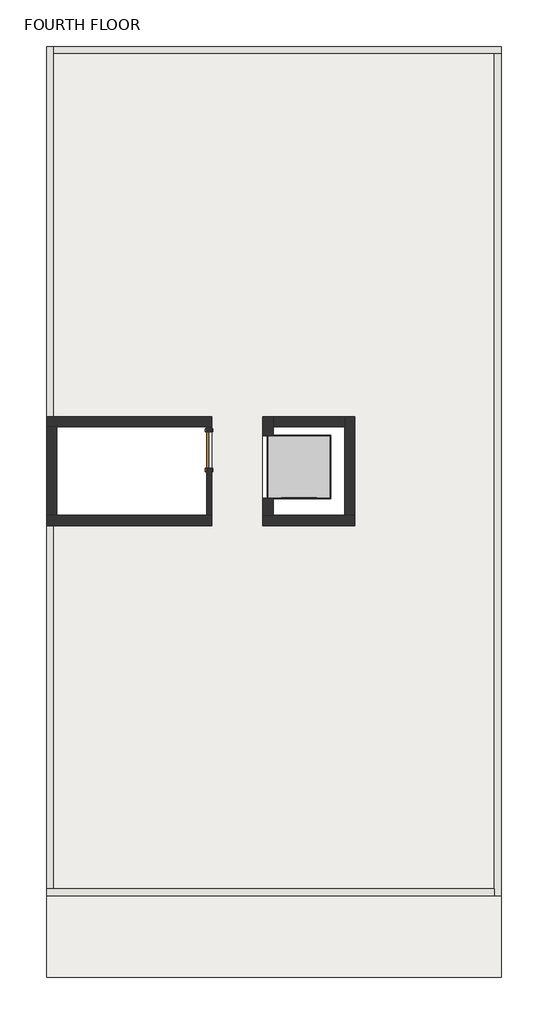
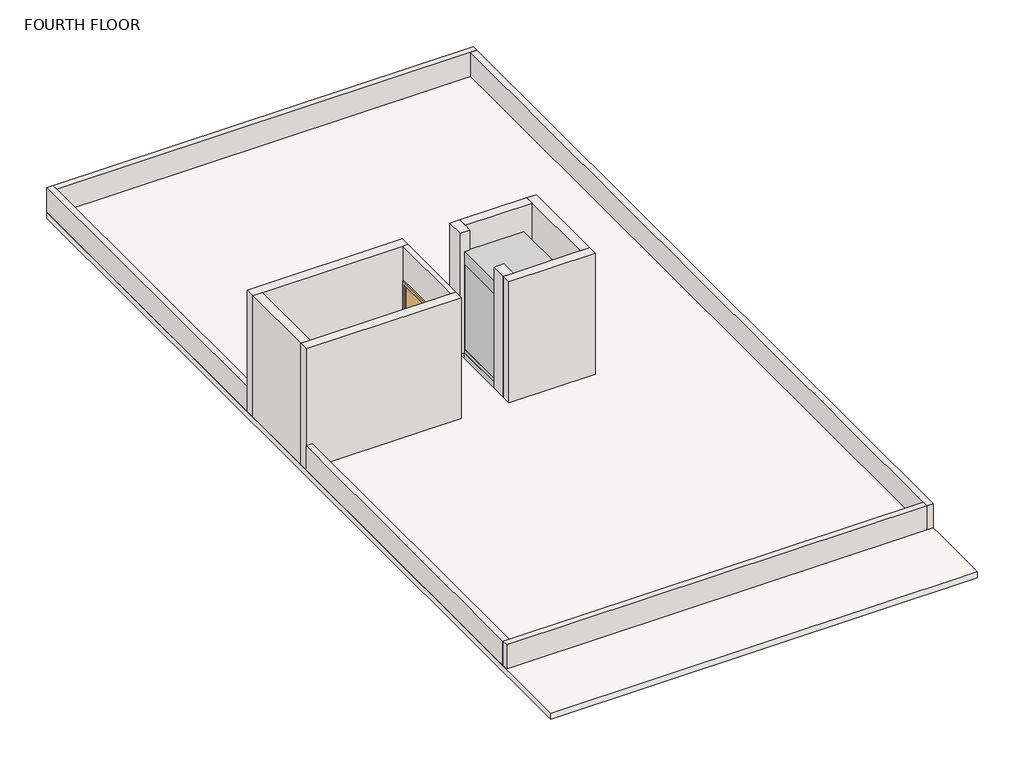
# One storey, incomplete: 14 walls, 1 door, 1 proxy, 1 slab.
"""IFC4 building model written with IfcOpenShell, lengths in millimetres."""

from ifc_helpers import new_model, si_unit, frame, origin, place, context, project, spatial, polyline, outline, extrude, faceted_brep, transform, mapped, element, save
from components import lift_glass_2_lift_with_hydraulic_ram_a28bd677, door_d141acb4

model = new_model("IFC4")

# Units and contexts
model_context = context("Model", 3, world=origin())
ifc_project = project(units=[si_unit("LENGTHUNIT", "METRE", prefix="MILLI")], contexts=[model_context])

# Site, building, storey
site = spatial("IfcSite", under=ifc_project)
building = spatial("IfcBuilding", under=site)
storey = spatial("IfcBuildingStorey", under=building, Name="FOURTH FLOOR", Elevation=12801.6)

# Proxy
placement = place(None, origin())
lift_glass_2_lift_with_hydraulic_ram_shape = lift_glass_2_lift_with_hydraulic_ram_a28bd677(model_context)
element("IfcBuildingElementProxy", 1, Name="Lift Glass (2) : Lift with Hydraulic Ram", ObjectType="Lift Glass (2) : Lift with Hydraulic Ram", at=placement, inside=storey, context=model_context, shape_type="MappedRepresentation", body=[
    mapped(lift_glass_2_lift_with_hydraulic_ram_shape, transform((-743.7147577, 597.8900134, 12801.6), x_axis=(1.0, 0.0, 0.0), y_axis=(0.0, 1.0, 0.0), z_axis=(0.0, 0.0, 1.0))),
])

# Door
door_shape = door_d141acb4(model_context)
element("IfcDoor", 2, ObjectType="Single-Flush : 2'8\"X7'", at=placement, inside=storey, context=model_context, shape_type="MappedRepresentation", body=[
    mapped(door_shape, transform((-2719.6789041, 1029.1153263, 12801.6), x_axis=(0.0, 1.0, 0.0), y_axis=(-1.0, 0.0, 0.0), z_axis=(0.0, 0.0, 1.0))),
])

# Slab
element("IfcSlab", 3, ObjectType="6\"", at=placement, inside=storey, context=model_context, shape_type="SweptSolid", body=[
    extrude(outline(polyline([(3814.4710959, 10058.8153263), (3814.4710959, -10769.1846737), (-6358.2289041, -10769.1846737), (-6358.2289041, 10058.8153263), (3814.4710959, 10058.8153263)]), holes=[polyline([(-2662.5289041, 1549.8153263), (-6129.6289041, 1549.8153263), (-6129.6289041, -431.3846737), (-2662.5289041, -431.3846737), (-2662.5289041, 1549.8153263)]), polyline([(537.8710959, 1778.4153263), (-1519.5289041, 1778.4153263), (-1519.5289041, -659.9846737), (537.8710959, -659.9846737), (537.8710959, 1778.4153263)])]), frame((0.0, 0.0, 12649.2), z_axis=(0.0, 0.0, 1.0), x_axis=(1.0, 0.0, 0.0)), (0.0, 0.0, 1.0), 152.4),
])

# Walls
element("IfcWall", 4, ObjectType="4.5\"", at=placement, inside=storey, context=model_context, shape_type="SweptSolid", body=[
    extrude(outline(polyline([(1549.8153263, 12801.6), (1435.5153263, 12801.6), (1435.5153263, 14935.2), (622.7153263, 14935.2), (622.7153263, 12801.6), (-431.3846737, 12801.6), (-431.3846737, 15849.6), (1549.8153263, 15849.6), (1549.8153263, 12801.6)])), frame((-2776.8289041, 0.0, 0.0), z_axis=(1.0, 0.0, 0.0), x_axis=(0.0, 1.0, 0.0)), (0.0, 0.0, 1.0), 114.3),
])
element("IfcWall", 5, ObjectType="6\"", at=placement, inside=storey, context=model_context, shape_type="Brep", body=[
    faceted_brep([(-6205.8289041, 1778.4153263, 12801.6), (-6205.8289041, 9906.4153263, 12801.6), (-6205.8289041, 10058.8153263, 12801.6), (-6205.8289041, 10058.8153263, 13411.2), (-6205.8289041, 9906.4153263, 13411.2), (-6205.8289041, 1778.4153263, 13411.2), (-6358.2289041, 1778.4153263, 12801.6), (-6358.2289041, 1778.4153263, 13411.2), (-6358.2289041, 10058.8153263, 13411.2), (-6358.2289041, 10058.8153263, 12801.6)], [[[0, 1, 2, 3, 4, 5]], [[6, 7, 8, 9]], [[2, 1, 0, 6, 9]], [[5, 4, 3, 8, 7]], [[0, 5, 7, 6]], [[3, 2, 9, 8]]]),
])
element("IfcWall", 6, ObjectType="6\"", at=placement, inside=storey, context=model_context, shape_type="Brep", body=[
    faceted_brep([(-6205.8289041, 9906.4153263, 12801.6), (3662.0710959, 9906.4153263, 12801.6), (3814.4710959, 9906.4153263, 12801.6), (3814.4710959, 9906.4153263, 13411.2), (3662.0710959, 9906.4153263, 13411.2), (-6205.8289041, 9906.4153263, 13411.2), (-6205.8289041, 10058.8153263, 12801.6), (-6205.8289041, 10058.8153263, 13411.2), (3814.4710959, 10058.8153263, 13411.2), (3814.4710959, 10058.8153263, 12801.6)], [[[0, 1, 2, 3, 4, 5]], [[6, 7, 8, 9]], [[2, 1, 0, 6, 9]], [[5, 4, 3, 8, 7]], [[0, 5, 7, 6]], [[3, 2, 9, 8]]]),
])
element("IfcWall", 7, ObjectType="6\"", at=placement, inside=storey, context=model_context, shape_type="Brep", body=[
    faceted_brep([(3662.0710959, 9906.4153263, 12801.6), (3662.0710959, -8787.9846737, 12801.6), (3662.0710959, -8940.3846737, 12801.6), (3662.0710959, -8940.3846737, 13411.2), (3662.0710959, -8787.9846737, 13411.2), (3662.0710959, 9906.4153263, 13411.2), (3814.4710959, 9906.4153263, 12801.6), (3814.4710959, 9906.4153263, 13411.2), (3814.4710959, -8940.3846737, 13411.2), (3814.4710959, -8940.3846737, 12801.6)], [[[0, 1, 2, 3, 4, 5]], [[6, 7, 8, 9]], [[2, 1, 0, 6, 9]], [[5, 4, 3, 8, 7]], [[0, 5, 7, 6]], [[3, 2, 9, 8]]]),
])
element("IfcWall", 8, ObjectType="6\"", at=placement, inside=storey, context=model_context, shape_type="Brep", body=[
    faceted_brep([(3662.0710959, -8787.9846737, 12801.6), (-6205.8289041, -8787.9846737, 12801.6), (-6358.2289041, -8787.9846737, 12801.6), (-6358.2289041, -8787.9846737, 13411.2), (-6205.8289041, -8787.9846737, 13411.2), (3662.0710959, -8787.9846737, 13411.2), (3662.0710959, -8940.3846737, 12801.6), (3662.0710959, -8940.3846737, 13411.2), (-6358.2289041, -8940.3846737, 13411.2), (-6358.2289041, -8940.3846737, 12801.6)], [[[0, 1, 2, 3, 4, 5]], [[6, 7, 8, 9]], [[2, 1, 0, 6, 9]], [[5, 4, 3, 8, 7]], [[0, 5, 7, 6]], [[3, 2, 9, 8]]]),
])
element("IfcWall", 9, ObjectType="6\"", at=placement, inside=storey, context=model_context, shape_type="SweptSolid", body=[
    extrude(outline(polyline([(-6205.8289041, -659.9846737), (-6205.8289041, -8787.9846737), (-6358.2289041, -8787.9846737), (-6358.2289041, -659.9846737), (-6205.8289041, -659.9846737)])), frame((0.0, 0.0, 12801.6), z_axis=(0.0, 0.0, 1.0), x_axis=(1.0, 0.0, 0.0)), (0.0, 0.0, 1.0), 609.6),
])
element("IfcWall", 10, ObjectType="9\"", at=placement, inside=storey, context=model_context, shape_type="Brep", body=[
    faceted_brep([(-2662.5289041, 1778.4153263, 12801.6), (-6205.8289041, 1778.4153263, 12801.6), (-6358.2289041, 1778.4153263, 12801.6), (-6358.2289041, 1778.4153263, 13411.2), (-6358.2289041, 1778.4153263, 15849.6), (-2662.5289041, 1778.4153263, 15849.6), (-2662.5289041, 1549.8153263, 12801.6), (-2662.5289041, 1549.8153263, 15849.6), (-2776.8289041, 1549.8153263, 15849.6), (-6129.6289041, 1549.8153263, 15849.6), (-6358.2289041, 1549.8153263, 15849.6), (-6358.2289041, 1549.8153263, 12801.6), (-6129.6289041, 1549.8153263, 12801.6), (-2776.8289041, 1549.8153263, 12801.6)], [[[0, 1, 2, 3, 4, 5]], [[6, 7, 8, 9, 10, 11, 12, 13]], [[2, 1, 0, 6, 13, 12, 11]], [[5, 4, 10, 9, 8, 7]], [[0, 5, 7, 6]], [[2, 11, 10, 4, 3]]]),
])
element("IfcWall", 11, ObjectType="9\"", at=placement, inside=storey, context=model_context, shape_type="Brep", body=[
    faceted_brep([(-2662.5289041, -431.3846737, 12801.6), (-2776.8289041, -431.3846737, 12801.6), (-6129.6289041, -431.3846737, 12801.6), (-6358.2289041, -431.3846737, 12801.6), (-6358.2289041, -431.3846737, 15849.6), (-6129.6289041, -431.3846737, 15849.6), (-2776.8289041, -431.3846737, 15849.6), (-2662.5289041, -431.3846737, 15849.6), (-2662.5289041, -659.9846737, 12801.6), (-2662.5289041, -659.9846737, 15849.6), (-6358.2289041, -659.9846737, 15849.6), (-6358.2289041, -659.9846737, 13411.2), (-6358.2289041, -659.9846737, 12801.6), (-6205.8289041, -659.9846737, 12801.6)], [[[0, 1, 2, 3, 4, 5, 6, 7]], [[8, 9, 10, 11, 12, 13]], [[3, 2, 1, 0, 8, 13, 12]], [[7, 6, 5, 4, 10, 9]], [[0, 7, 9, 8]], [[3, 12, 11, 10, 4]]]),
])
element("IfcWall", 12, ObjectType="9\"", at=placement, inside=storey, context=model_context, shape_type="SweptSolid", body=[
    extrude(outline(polyline([(-6358.2289041, -431.3846737), (-6358.2289041, 1549.8153263), (-6129.6289041, 1549.8153263), (-6129.6289041, -431.3846737), (-6358.2289041, -431.3846737)])), frame((0.0, 0.0, 12801.6), z_axis=(0.0, 0.0, 1.0), x_axis=(1.0, 0.0, 0.0)), (0.0, 0.0, 1.0), 3048.0),
])
element("IfcWall", 13, ObjectType="9\"", at=placement, inside=storey, context=model_context, shape_type="Brep", body=[
    faceted_brep([(-1519.5289041, -659.9846737, 12801.6), (537.8710959, -659.9846737, 12801.6), (537.8710959, -659.9846737, 15849.6), (-1519.5289041, -659.9846737, 15849.6), (-1519.5289041, -431.3846737, 12801.6), (-1519.5289041, -431.3846737, 15849.6), (-1290.9289041, -431.3846737, 15849.6), (309.2710959, -431.3846737, 15849.6), (537.8710959, -431.3846737, 15849.6), (537.8710959, -431.3846737, 12801.6), (309.2710959, -431.3846737, 12801.6), (-1290.9289041, -431.3846737, 12801.6)], [[[0, 1, 2, 3]], [[4, 5, 6, 7, 8, 9, 10, 11]], [[1, 0, 4, 11, 10, 9]], [[3, 2, 8, 7, 6, 5]], [[2, 1, 9, 8]], [[0, 3, 5, 4]]]),
])
element("IfcWall", 14, ObjectType="9\"", at=placement, inside=storey, context=model_context, shape_type="Brep", body=[
    faceted_brep([(537.8710959, -431.3846737, 12801.6), (537.8710959, 1778.4153263, 12801.6), (537.8710959, 1778.4153263, 15849.6), (537.8710959, -431.3846737, 15849.6), (309.2710959, -431.3846737, 12801.6), (309.2710959, -431.3846737, 15849.6), (309.2710959, 1549.8153263, 15849.6), (309.2710959, 1778.4153263, 15849.6), (309.2710959, 1778.4153263, 12801.6), (309.2710959, 1549.8153263, 12801.6)], [[[0, 1, 2, 3]], [[4, 5, 6, 7, 8, 9]], [[1, 0, 4, 9, 8]], [[3, 2, 7, 6, 5]], [[0, 3, 5, 4]], [[2, 1, 8, 7]]]),
])
element("IfcWall", 15, ObjectType="9\"", at=placement, inside=storey, context=model_context, shape_type="SweptSolid", body=[
    extrude(outline(polyline([(309.2710959, 1549.8153263), (-1290.9289041, 1549.8153263), (-1290.9289041, 1778.4153263), (309.2710959, 1778.4153263), (309.2710959, 1549.8153263)])), frame((0.0, 0.0, 12801.6), z_axis=(0.0, 0.0, 1.0), x_axis=(1.0, 0.0, 0.0)), (0.0, 0.0, 1.0), 3048.0),
])
element("IfcWall", 16, ObjectType="9\"", at=placement, inside=storey, context=model_context, shape_type="Brep", body=[
    faceted_brep([(-1519.5289041, 1778.4153263, 12801.6), (-1519.5289041, 1349.8153263, 12801.6), (-1519.5289041, 1349.8153263, 15849.6), (-1519.5289041, 1778.4153263, 15849.6), (-1290.9289041, 1778.4153263, 12801.6), (-1290.9289041, 1778.4153263, 15849.6), (-1290.9289041, 1549.8153263, 15849.6), (-1290.9289041, 1349.8153263, 15849.6), (-1290.9289041, 1349.8153263, 12801.6), (-1290.9289041, 1549.8153263, 12801.6)], [[[0, 1, 2, 3]], [[4, 5, 6, 7, 8, 9]], [[1, 0, 4, 9, 8]], [[2, 1, 8, 7]], [[3, 2, 7, 6, 5]], [[0, 3, 5, 4]]]),
])
element("IfcWall", 17, ObjectType="9\"", at=placement, inside=storey, context=model_context, shape_type="SweptSolid", body=[
    extrude(outline(polyline([(-1290.9289041, -50.1846737), (-1290.9289041, -431.3846737), (-1519.5289041, -431.3846737), (-1519.5289041, -50.1846737), (-1290.9289041, -50.1846737)])), frame((0.0, 0.0, 12801.6), z_axis=(0.0, 0.0, 1.0), x_axis=(1.0, 0.0, 0.0)), (0.0, 0.0, 1.0), 3048.0),
])

save(model, "model.ifc")

# Revit data of these elements
# Type "Lift Glass (2) : Lift with Hydraulic Ram"
#   Stile Top Rail = 0' - 3.93701"
#   Stile Shutting = 0' - 1.9685"
#   Stile Hanging Rail = 0' - 1.9685"
#   Stile Bottom = 0' - 3.93701"
#   Skirting Ht = 0' - 3.93701"
#   Hoistway Depth = 5' - 10.86614"
#   Hoistway Width = 6' - 2.80315"
#   Roof Thickness = 0' - 9.84252"
#   Lift Car Width = 4' - 7.11811"
#   Lift Rise = 4' - 11.05512"
#   Lift Height = 7' - 6.55118"
#   Lift Car Depth = 4' - 7.11811"
#   Glazing Thickness = 0' - 0.47244"
#   Floor Thickness = 0' - 11.81102"
#   Floor Offset = 0' - 0.47244"
#   Door Opening = 2' - 7.49606"
#   Door Offset = 0' - 0.98425"
#   Cornice Ht = 0' - 2.95276"
#   Vis - Hydraulic Ram = yes
#   Vis - Hoistway Placement Lines = yes
#   Material Solid panel = Stainless Steel
#   Material Lift Car = Stainless Steel
#   Material Glass = Glass
#   Default Elevation = 0
# Type "Single-Flush : 2'8\"X7'"
#   Type Mark = "12"
#   Construction Type Id = "MDOOR"
#   Assembly Code = "C1020"
#   Analytic Construction = "Metal"
#   Thickness = 0' - 2"
#   Heat Transfer Coefficient (U) = 0.651978 BTU/(h·ft²·°F)
#   Height = 7' - 0"
#   Trim Projection Ext = 0' - 1"
#   Trim Projection Int = 0' - 1"
#   Trim Width = 0' - 3"
#   Width = 2' - 8"
#   Define Thermal Properties by = 1
#   Door Material = Door - Panel
#   Frame Material = Door - Frame
#   Visual Light Transmittance = 0
#   Solar Heat Gain Coefficient = 0
#   Function = (empty or 0)
#   Wall Closure = (empty or 0)
# Type "6\""
#   Assembly Code = "B1010"
#   Function = 0
#   Layers, outside or top first: 0' - 6" no material (function 1)
# Type "4.5\""
#   Assembly Code = "B2010"
#   Layers, outside or top first: 0' - 4 1/2" no material (function 1)
# Type "6\""
#   Assembly Code = "B2010"
#   Layers, outside or top first: 0' - 6" no material (function 1)
# Type "9\""
#   Assembly Code = "B2010"
#   Layers, outside or top first: 0' - 9" "WALL" (function 1)
# Element 1 (IfcBuildingElementProxy, "Lift Glass (2) : Lift with Hydraulic Ram")
#   Phase Created = New Construction
#   Materials on its faces: "Stainless Steel", "Glass", "Paint - Green"
# Element 2 (IfcDoor, "Single-Flush : 2'8\"X7'")
#   Phase Created = New Construction
#   Materials on its faces: "Door - Frame", "Door - Panel"
# Element 3 (IfcSlab, "6\"")
#   Height Offset From Level = 0' - 0"
#   Phase Created = New Construction
#   Materials on its faces: "Default Floor", "DUSTY ROSE"
# Element 4 (IfcWall, "4.5\"")
#   Top Offset = 10' - 0"
#   Base Offset = 0' - 0"
#   wall height = 10' - 0"
#   Phase Created = New Construction
#   Base Constraint = FOURTH FLOOR
#   Top Constraint = FOURTH FLOOR
#   Materials on its faces: "Default Wall"
# Elements 5, 6 (IfcWall, "6\"")
#   Top Offset = -0' - 6"
#   Base Offset = 0' - 0"
#   Unconnected Height = 2' - 0"
#   wall height = 2' - 0"
#   Phase Created = New Construction
#   Base Constraint = FOURTH FLOOR
#   Materials on its faces: "6\" WALL", "Default Wall"
# Elements 7, 8, 9 (IfcWall, "6\"")
#   Top Offset = -0' - 6"
#   Base Offset = 0' - 0"
#   Unconnected Height = 2' - 0"
#   wall height = 2' - 0"
#   Phase Created = New Construction
#   Base Constraint = FOURTH FLOOR
#   Materials on its faces: "Default Wall", "6\" WALL"
# Elements 10, 11 (IfcWall, "9\"")
#   Top Offset = 10' - 0"
#   Base Offset = 0' - 0"
#   wall height = 10' - 0"
#   Phase Created = New Construction
#   Base Constraint = FOURTH FLOOR
#   Top Constraint = FOURTH FLOOR
#   Materials on its faces: "WALL", "Default Wall", "6\" WALL"
# Element 12 (IfcWall, "9\"")
#   Top Offset = 10' - 0"
#   Base Offset = 0' - 0"
#   wall height = 10' - 0"
#   Phase Created = New Construction
#   Base Constraint = FOURTH FLOOR
#   Top Constraint = FOURTH FLOOR
#   Materials on its faces: "WALL", "6\" WALL"
# Elements 13, 14, 15, 16, 17 (IfcWall, "9\"")
#   Top Offset = -0' - 6"
#   Base Offset = 0' - 0"
#   wall height = 10' - 0"
#   Phase Created = New Construction
#   Base Constraint = FOURTH FLOOR
#   Top Constraint = ROOF
#   Materials on its faces: "WALL"
# Materials
#   "Stainless Steel": class "Metal", colour RGB 0 0 0, transparency 0, Description = "Stainless Steel 18/8", Cost = 0
#   "Glass": class "Glass", colour RGB 0 128 192, transparency 0.75, Description = "Soda Lime Glass", Cost = 0
#   "Door - Panel": class "Wood", colour RGB 210 159 95, transparency 0, Cost = 0
#   "Door - Frame": colour RGB 118 70 51, transparency 0, Cost = 0
#   "WALL": class "Generic", colour RGB 84 102 113, transparency 0, Cost = 0
#   "Paint - Green": colour RGB 0 128 64, transparency 0
#   "Default Floor": colour RGB 128 128 128, transparency 0, Cost = 0
#   "DUSTY ROSE": class "Generic", colour RGB 120 120 120, transparency 0, Cost = 0
#   "Default Wall": colour RGB 128 128 128, transparency 0, Cost = 0
#   "6\" WALL": class "Generic", colour RGB 186 182 182, transparency 0, Cost = 0
